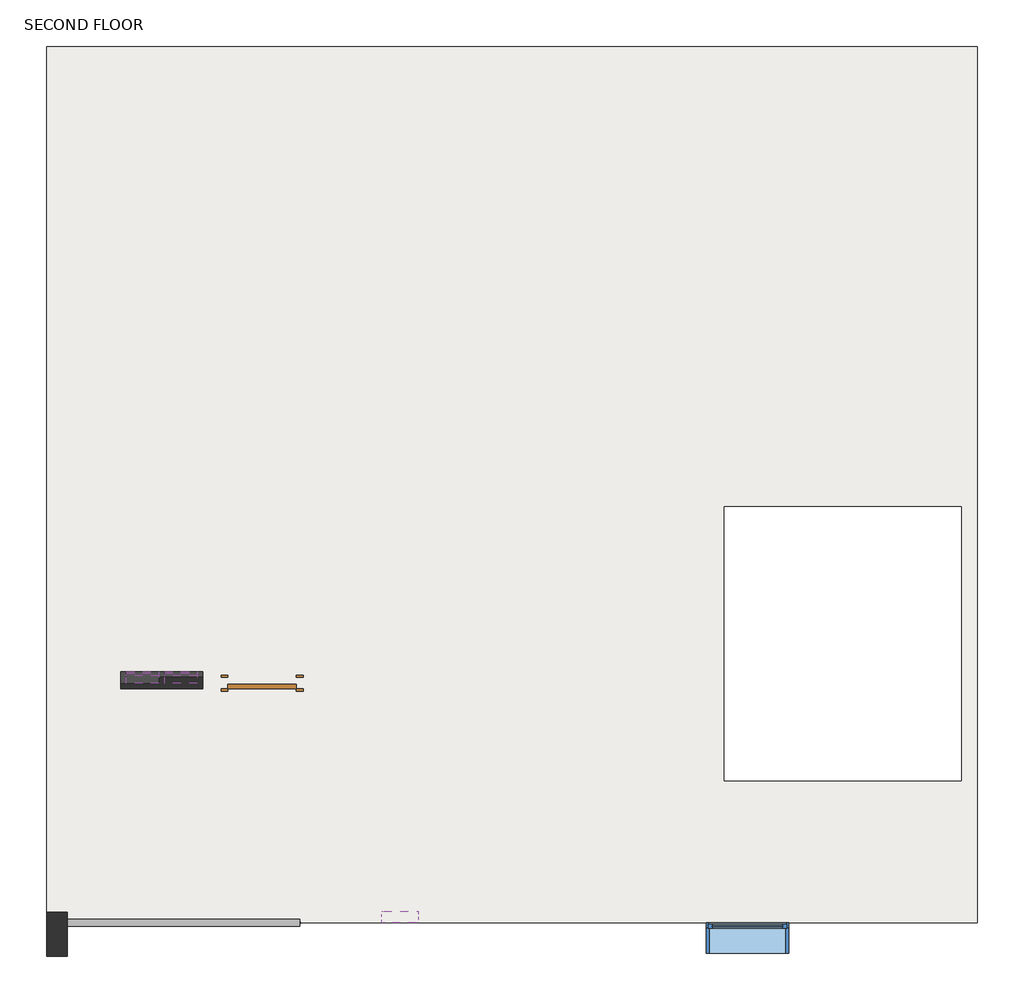
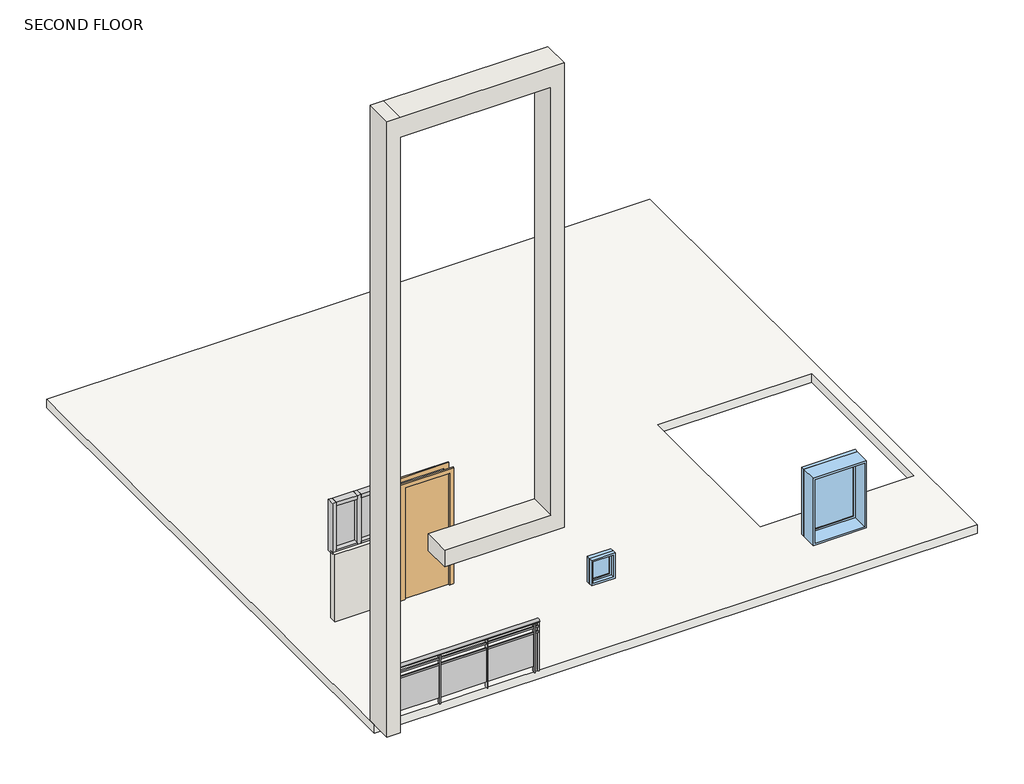
# One storey: 7 members, 2 plates, 2 walls, 2 windows, 1 door, 1 railing, 1 slab.
"""IFC4 building model written with IfcOpenShell, lengths in millimetres."""

from ifc_helpers import new_model, si_unit, point, frame, origin, place, context, project, spatial, polyline, ellipse_curve, trimmed, outline, extrude, transform, mapped, element, save
from ifc_brep_helpers import plane_surface, extruded_surface, advanced_brep
from components import door_e00f436c, member_d959a85f, member_843225dc, member_54f829b7, system_panel_glazed_8fc33089, walls_4_walls_4_370afa2d, fixed_bw_be0fa6e9, fixed_ven_0bde2124

model = new_model("IFC4")

# Units and contexts
model_context = context("Model", 3, world=origin())
ifc_project = project(units=[si_unit("LENGTHUNIT", "METRE", prefix="MILLI")], contexts=[model_context])

# Site, building, storey
site = spatial("IfcSite", under=ifc_project)
building = spatial("IfcBuilding", under=site)
storey = spatial("IfcBuildingStorey", under=building, Name="SECOND FLOOR", Elevation=6096.0)

# Door
placement = place(None, origin())
door_shape = door_e00f436c(model_context)
element("IfcDoor", 1, ObjectType="Single-Flush : 36\" x 84\"", at=placement, inside=storey, context=model_context, shape_type="MappedRepresentation", body=[
    mapped(door_shape, transform((-4124.5569651, 3118.5055142, 6096.0), x_axis=(1.0, 0.0, 0.0), y_axis=(0.0, 1.0, 0.0), z_axis=(0.0, 0.0, 1.0))),
])

# Members
member_shape = member_d959a85f(model_context)
element("IfcMember", 2, ObjectType="Rectangular Mullion : 2.5\" x 5\" rectangular", at=placement, inside=storey, context=model_context, shape_type="MappedRepresentation", body=[
    mapped(member_shape, transform((-4784.9569651, 3182.0055142, 7285.4584417), x_axis=(1.0, 0.0, 0.0), y_axis=(0.0, -1.0, 0.0), z_axis=(0.0, 0.0, -1.0))),
])
element("IfcMember", 3, ObjectType="Rectangular Mullion : 2.5\" x 5\" rectangular", at=placement, inside=storey, context=model_context, shape_type="MappedRepresentation", body=[
    mapped(member_shape, transform((-5699.3569651, 3182.0055142, 8204.2), x_axis=(-1.0, 0.0, 0.0), y_axis=(0.0, -1.0, 0.0), z_axis=(0.0, 0.0, 1.0))),
])
member_2_shape = member_843225dc(model_context)
element("IfcMember", 4, ObjectType="Rectangular Mullion : 2.5\" x 5\" rectangular", at=placement, inside=storey, context=model_context, shape_type="MappedRepresentation", body=[
    mapped(member_2_shape, transform((-4848.4569651, 3182.0055142, 8204.2), x_axis=(0.0, 0.0, 1.0), y_axis=(0.0, -1.0, 0.0), z_axis=(1.0, 0.0, 0.0))),
])
element("IfcMember", 5, ObjectType="Rectangular Mullion : 2.5\" x 5\" rectangular", at=placement, inside=storey, context=model_context, shape_type="MappedRepresentation", body=[
    mapped(member_2_shape, transform((-5273.9069651, 3182.0055142, 8204.2), x_axis=(0.0, 0.0, 1.0), y_axis=(0.0, -1.0, 0.0), z_axis=(1.0, 0.0, 0.0))),
])
element("IfcMember", 6, ObjectType="Rectangular Mullion : 2.5\" x 5\" rectangular", at=placement, inside=storey, context=model_context, shape_type="MappedRepresentation", body=[
    mapped(member_2_shape, transform((-5635.8569651, 3182.0055142, 7285.4584417), x_axis=(0.0, 0.0, -1.0), y_axis=(0.0, -1.0, 0.0), z_axis=(-1.0, 0.0, 0.0))),
])
element("IfcMember", 7, ObjectType="Rectangular Mullion : 2.5\" x 5\" rectangular", at=placement, inside=storey, context=model_context, shape_type="MappedRepresentation", body=[
    mapped(member_2_shape, transform((-5210.4069651, 3182.0055142, 7285.4584417), x_axis=(0.0, 0.0, -1.0), y_axis=(0.0, -1.0, 0.0), z_axis=(-1.0, 0.0, 0.0))),
])
member_3_shape = member_54f829b7(model_context)
element("IfcMember", 8, ObjectType="Rectangular Mullion : 2.5\" x 5\" rectangular", at=placement, inside=storey, context=model_context, shape_type="MappedRepresentation", body=[
    mapped(member_3_shape, transform((-5242.1569651, 3182.0055142, 7285.4584417), x_axis=(1.0, 0.0, 0.0), y_axis=(0.0, -1.0, 0.0), z_axis=(0.0, 0.0, -1.0))),
])

# Plates
system_panel_glazed_shape = system_panel_glazed_8fc33089(model_context)
element("IfcPlate", 9, ObjectType="System Panel : Glazed", at=placement, inside=storey, context=model_context, shape_type="MappedRepresentation", body=[
    mapped(system_panel_glazed_shape, transform((-5454.8819651, 3182.0055142, 7348.9584417), x_axis=(1.0, 0.0, 0.0), y_axis=(0.0, 1.0, 0.0), z_axis=(0.0, 0.0, 1.0))),
])
element("IfcPlate", 10, ObjectType="System Panel : Glazed", at=placement, inside=storey, context=model_context, shape_type="MappedRepresentation", body=[
    mapped(system_panel_glazed_shape, transform((-5029.4319651, 3182.0055142, 7348.9584417), x_axis=(1.0, 0.0, 0.0), y_axis=(0.0, 1.0, 0.0), z_axis=(0.0, 0.0, 1.0))),
])

# Railing
element("IfcRailing", 11, ObjectType="Glass Panel - Bottom Fill", at=placement, inside=storey, context=model_context, shape_type="SolidModel", body=[
    advanced_brep(
    [(-6296.2569651, 489.6055142, 7010.4), (-6296.2569651, 413.4055142, 7010.4), (-3705.4569651, 489.6055142, 7010.4), (-3705.4569651, 413.4055142, 7010.4)],
    [
        (0, 1, ellipse_curve(frame((-6296.2569651, 451.5055142, 7010.4), z_axis=(-1.0, 0.0, 0.0), x_axis=(0.0, -1.0, 0.0)), 38.1, 28.575)),
        (1, 0, ellipse_curve(frame((-6296.2569651, 451.5055142, 7010.4), z_axis=(-1.0, 0.0, 0.0), x_axis=(0.0, -1.0, 0.0)), 38.1, 28.575)),
        (2, 3, ellipse_curve(frame((-3705.4569651, 451.5055142, 7010.4), z_axis=(1.0, 0.0, 0.0), x_axis=(0.0, -1.0, 0.0)), 38.1, 28.575)),
        (3, 2, ellipse_curve(frame((-3705.4569651, 451.5055142, 7010.4), z_axis=(1.0, 0.0, 0.0), x_axis=(0.0, -1.0, 0.0)), 38.1, 28.575)),
        (0, 2),
        (3, 1),
    ],
    [
        plane_surface(frame((-6296.2569651, 451.5055142, 7010.4), z_axis=(-1.0, 0.0, 0.0), x_axis=(0.0, 1.0, 0.0))),
        plane_surface(frame((-3705.4569651, 451.5055142, 7010.4), z_axis=(1.0, 0.0, 0.0), x_axis=(0.0, 1.0, 0.0))),
        extruded_surface(trimmed(ellipse_curve(frame((-3705.4569651, 451.5055142, 7010.4), z_axis=(-1.0, 0.0, 0.0), x_axis=(0.0, -1.0, 0.0)), 38.1, 28.575), [point((-3705.4569651, 489.6055142, 7010.4))], [point((-3705.4569651, 413.4055142, 7010.4))], True, "CARTESIAN"), (-2590.8, 0.0, 0.0), 2590.8),
        extruded_surface(trimmed(ellipse_curve(frame((-3705.4569651, 451.5055142, 7010.4), z_axis=(-1.0, 0.0, 0.0), x_axis=(0.0, -1.0, 0.0)), 38.1, 28.575), [point((-3705.4569651, 413.4055142, 7010.4))], [point((-3705.4569651, 489.6055142, 7010.4))], True, "CARTESIAN"), (-2590.8, 0.0, 0.0), 2590.8),
    ],
    [
        (0, [[1, 2]]),
        (1, [[3, 4]]),
        (2, [[-1, 5, -4, 6]]),
        (3, [[-2, -6, -3, -5]]),
    ],
),
    extrude(outline(polyline([(-6296.2569651, 438.8055142), (-6296.2569651, 464.2055142), (-3705.4569651, 464.2055142), (-3705.4569651, 438.8055142), (-6296.2569651, 438.8055142)])), frame((0.0, 0.0, 6896.1), z_axis=(0.0, 0.0, 1.0), x_axis=(1.0, 0.0, 0.0)), (0.0, 0.0, 1.0), 25.4),
    extrude(outline(polyline([(-6296.2569651, 438.8055142), (-6296.2569651, 464.2055142), (-3705.4569651, 464.2055142), (-3705.4569651, 438.8055142), (-6296.2569651, 438.8055142)])), frame((0.0, 0.0, 6794.5), z_axis=(0.0, 0.0, 1.0), x_axis=(1.0, 0.0, 0.0)), (0.0, 0.0, 1.0), 25.4),
    extrude(outline(polyline([(-3788.0069651, 426.1055142), (-3788.0069651, 476.9055142), (-3775.3069651, 476.9055142), (-3775.3069651, 426.1055142), (-3788.0069651, 426.1055142)])), frame((0.0, 0.0, 6096.0), z_axis=(0.0, 0.0, 1.0), x_axis=(1.0, 0.0, 0.0)), (0.0, 0.0, 1.0), 885.6788223),
    extrude(outline(polyline([(-4594.4569651, 458.0406712), (-3781.6569651, 458.0406712), (-3781.6569651, 451.6906712), (-4594.4569651, 451.6906712), (-4594.4569651, 458.0406712)])), frame((0.0, 0.0, 6197.6), z_axis=(0.0, 0.0, 1.0), x_axis=(1.0, 0.0, 0.0)), (0.0, 0.0, 1.0), 596.9),
    extrude(outline(polyline([(-4600.8069651, 426.1055142), (-4600.8069651, 476.9055142), (-4588.1069651, 476.9055142), (-4588.1069651, 426.1055142), (-4600.8069651, 426.1055142)])), frame((0.0, 0.0, 6096.0), z_axis=(0.0, 0.0, 1.0), x_axis=(1.0, 0.0, 0.0)), (0.0, 0.0, 1.0), 885.6788223),
    extrude(outline(polyline([(-5407.2569651, 458.0406712), (-4594.4569651, 458.0406712), (-4594.4569651, 451.6906712), (-5407.2569651, 451.6906712), (-5407.2569651, 458.0406712)])), frame((0.0, 0.0, 6197.6), z_axis=(0.0, 0.0, 1.0), x_axis=(1.0, 0.0, 0.0)), (0.0, 0.0, 1.0), 596.9),
    extrude(outline(polyline([(-5413.6069651, 426.1055142), (-5413.6069651, 476.9055142), (-5400.9069651, 476.9055142), (-5400.9069651, 426.1055142), (-5413.6069651, 426.1055142)])), frame((0.0, 0.0, 6096.0), z_axis=(0.0, 0.0, 1.0), x_axis=(1.0, 0.0, 0.0)), (0.0, 0.0, 1.0), 885.6788223),
    extrude(outline(polyline([(-6220.0569651, 458.0406712), (-5407.2569651, 458.0406712), (-5407.2569651, 451.6906712), (-6220.0569651, 451.6906712), (-6220.0569651, 458.0406712)])), frame((0.0, 0.0, 6197.6), z_axis=(0.0, 0.0, 1.0), x_axis=(1.0, 0.0, 0.0)), (0.0, 0.0, 1.0), 596.9),
    extrude(outline(polyline([(-6226.4069651, 426.1055142), (-6226.4069651, 476.9055142), (-6213.7069651, 476.9055142), (-6213.7069651, 426.1055142), (-6226.4069651, 426.1055142)])), frame((0.0, 0.0, 6096.0), z_axis=(0.0, 0.0, 1.0), x_axis=(1.0, 0.0, 0.0)), (0.0, 0.0, 1.0), 885.6788223),
    extrude(outline(polyline([(-3718.1569651, 441.9805142), (-3718.1569651, 461.0305142), (-3699.1069651, 461.0305142), (-3699.1069651, 441.9805142), (-3718.1569651, 441.9805142)])), frame((0.0, 0.0, 6096.0), z_axis=(0.0, 0.0, 1.0), x_axis=(1.0, 0.0, 0.0)), (0.0, 0.0, 1.0), 885.6788223),
    extrude(outline(polyline([(-6302.6069651, 441.9805142), (-6302.6069651, 461.0305142), (-6283.5569651, 461.0305142), (-6283.5569651, 441.9805142), (-6302.6069651, 441.9805142)])), frame((0.0, 0.0, 6096.0), z_axis=(0.0, 0.0, 1.0), x_axis=(1.0, 0.0, 0.0)), (0.0, 0.0, 1.0), 885.6788223),
])

# Slab
element("IfcSlab", 12, ObjectType="Generic - 12\"", at=placement, inside=storey, context=model_context, shape_type="SweptSolid", body=[
    extrude(outline(polyline([(3838.3430349, 10205.1055142), (3838.3430349, 451.5055142), (-6524.8569651, 451.5055142), (-6524.8569651, 10205.1055142), (3838.3430349, 10205.1055142)]), holes=[polyline([(3660.5430349, 5080.6555142), (1018.9430349, 5080.6555142), (1018.9430349, 2032.6555142), (3660.5430349, 2032.6555142), (3660.5430349, 5080.6555142)])]), frame((0.0, 0.0, 5943.6), z_axis=(0.0, 0.0, 1.0), x_axis=(1.0, 0.0, 0.0)), (0.0, 0.0, 1.0), 152.4),
])

# Walls
element("IfcWall", 13, ObjectType="5\"", at=placement, inside=storey, context=model_context, shape_type="SweptSolid", body=[
    extrude(outline(polyline([(-4784.9569651, 3055.0055142), (-5699.3569651, 3055.0055142), (-5699.3569651, 3182.0055142), (-4784.9569651, 3182.0055142), (-4784.9569651, 3055.0055142)])), frame((0.0, 0.0, 5156.2), z_axis=(0.0, 0.0, 1.0), x_axis=(1.0, 0.0, 0.0)), (0.0, 0.0, 1.0), 2159.0),
])
walls_4_walls_4_shape = walls_4_walls_4_370afa2d(model_context)
element("IfcWall", 14, ObjectType="Walls 4 : Walls 4", at=placement, inside=storey, context=model_context, shape_type="MappedRepresentation", body=[
    mapped(walls_4_walls_4_shape, transform((0.0, 0.0, 0.0), x_axis=(1.0, 0.0, 0.0), y_axis=(0.0, 1.0, 0.0), z_axis=(0.0, 0.0, 1.0))),
])

# Windows
fixed_bw_shape = fixed_bw_be0fa6e9(model_context)
element("IfcWindow", 15, ObjectType="Fixed : BW", at=placement, inside=storey, context=model_context, shape_type="MappedRepresentation", body=[
    mapped(fixed_bw_shape, transform((1316.0073388, 281.3921573, 6070.6), x_axis=(1.0, 0.0, 0.0), y_axis=(0.0, 1.0, 0.0), z_axis=(0.0, 0.0, 1.0))),
])
fixed_ven_shape = fixed_ven_0bde2124(model_context)
element("IfcWindow", 16, ObjectType="Fixed : VEN", at=placement, inside=storey, context=model_context, shape_type="MappedRepresentation", body=[
    mapped(fixed_ven_shape, transform((-2549.7569651, 515.0055142, 6397.0646104), x_axis=(1.0, 0.0, 0.0), y_axis=(0.0, 1.0, 0.0), z_axis=(0.0, 0.0, 1.0))),
])

save(model, "model.ifc")

# Revit data of these elements
# Type "Single-Flush : 36\" x 84\""
#   Type Mark = "1"
#   Construction Type Id = "MDOOR"
#   Assembly Code = "C1020"
#   Analytic Construction = "Metal"
#   Thickness = 0' - 2"
#   Heat Transfer Coefficient (U) = 0.651978 BTU/(h·ft²·°F)
#   Height = 6' - 8"
#   Trim Projection Ext = 0' - 1"
#   Trim Projection Int = 0' - 1"
#   Trim Width = 0' - 3"
#   Width = 2' - 6"
#   Define Thermal Properties by = 1
#   Define Thermal Properties by = 1
#   Door Material = Door - Panel
#   Frame Material = Door - Frame
#   Visual Light Transmittance = 0
#   Solar Heat Gain Coefficient = 0
#   Function = (empty or 0)
#   Wall Closure = (empty or 0)
# Type "Rectangular Mullion : 2.5\" x 5\" rectangular"
#   built-in parameter 1007304 = 0.416667 (stored number, unit not read)
#   built-in parameter 1007301 = 0.104167 (stored number, unit not read)
#   built-in parameter 1007300 = 0.104167 (stored number, unit not read)
# Type "System Panel : Glazed"
#   Construction Type Id = "GSP4R"
#   Analytic Construction = "1/8 in Pilkington single glazing"
#   Visual Light Transmittance = 0.9
#   Solar Heat Gain Coefficient = 0.86
#   Heat Transfer Coefficient (U) = 1.18115 BTU/(h·ft²·°F)
#   Define Thermal Properties by = 1
# Type "Glass Panel - Bottom Fill"
#   Assembly Code = "C2010400"
#   built-in parameter 1008612 = 0.0416667 (stored number, unit not read)
#   built-in parameter 1008611 = 0.0416667 (stored number, unit not read)
#   built-in parameter 1008609 = 0.333333 (stored number, unit not read)
#   built-in parameter 1008604 = 0.166667 (stored number, unit not read)
#   built-in parameter 1008603 = 0.166667 (stored number, unit not read)
#   Railing Height = 3' - 0"
#   built-in parameter 1008630 = 2
#   built-in parameter 1008610 = 2
#   built-in parameter 1008618 = Baluster - Square : 3/4"
# Type "Generic - 12\""
#   Assembly Code = "B1010"
#   Function = 0
#   Layers, outside or top first: 0' - 6" no material (function 1)
# Type "5\""
#   Assembly Code = "B2010"
#   Layers, outside or top first: 0' - 5" "Concrete Masonry Units" (function 1)
# Type "Fixed : BW"
#   Type Mark = "18"
#   Construction Type Id = "GSP4R"
#   Assembly Code = "B2020100"
#   Analytic Construction = "1/8 in Pilkington single glazing"
#   Visual Light Transmittance = 0.9
#   Solar Heat Gain Coefficient = 0.78
#   Heat Transfer Coefficient (U) = 0.6496 BTU/(h·ft²·°F)
#   Height = 4' - 0"
#   Default Sill Height = 3' - 0"
#   Width = 3' - 0"
#   Window Inset = 0' - 0 3/4"
#   Define Thermal Properties by = 1
#   Glass Pane Material = Glass
#   Sash Material = Sash
#   Wall Closure = (empty or 0)
# Type "Fixed : VEN"
#   Type Mark = "19"
#   Construction Type Id = "GSP4R"
#   Assembly Code = "B2020100"
#   Analytic Construction = "1/8 in Pilkington single glazing"
#   Visual Light Transmittance = 0.9
#   Solar Heat Gain Coefficient = 0.78
#   Heat Transfer Coefficient (U) = 0.6496 BTU/(h·ft²·°F)
#   Height = 1' - 6"
#   Default Sill Height = 3' - 0"
#   Width = 1' - 4"
#   Window Inset = 0' - 0 3/4"
#   Define Thermal Properties by = 1
#   Glass Pane Material = Glass
#   Sash Material = Sash
#   Wall Closure = (empty or 0)
# Element 1 (IfcDoor, "Single-Flush : 36\" x 84\"")
#   Phase Created = New Construction
#   Materials on its faces: "Door - Frame", "Door - Panel"
# Elements 2, 3, 4, 5, 6, 7, 8 (IfcMember, "Rectangular Mullion : 2.5\" x 5\" rectangular")
#   Phase Created = New Construction
#   Materials on its faces: "Aluminum"
# Elements 9, 10 (IfcPlate, "System Panel : Glazed")
#   Phase Created = New Construction
#   Materials on its faces: "Glass"
# Element 11 (IfcRailing, "Glass Panel - Bottom Fill")
#   Phase Created = New Construction
#   Materials on its faces: "Glass"
# Element 12 (IfcSlab, "Generic - 12\"")
#   Height Offset From Level = 0' - 0"
#   Phase Created = New Construction
#   Materials on its faces: "Default Floor", "1 wall brown"
# Element 13 (IfcWall, "5\"")
#   built-in parameter 1001111 = -3' - 1"
#   Top Offset = 0' - 0"
#   Base Offset = -3' - 1"
#   Unconnected Height = 7' - 1"
#   wall height = 7' - 1"
#   Phase Created = New Construction
#   Base Constraint = SECOND FLOOR
#   Materials on its faces: "Concrete Masonry Units", "1 wall white"
# Element 14 (IfcWall, "Walls 4 : Walls 4")
#   Phase Created = New Construction
#   Materials on its faces: "1 wall brown", "Default Wall"
# Element 15 (IfcWindow, "Fixed : BW")
#   Mark = "8"
#   Phase Created = New Construction
#   Materials on its faces: "Sash", "Glass"
# Element 16 (IfcWindow, "Fixed : VEN")
#   Mark = "11"
#   Phase Created = New Construction
#   Materials on its faces: "Sash", "Glass"
# Materials
#   "Door - Panel": class "Wood", colour RGB 210 159 95, transparency 0, Cost = 0
#   "Door - Frame": colour RGB 118 70 51, transparency 0, Cost = 0
#   "Concrete Masonry Units": class "Masonry", colour RGB 227 227 227, transparency 0, Description = "Concrete masonry units", Cost = 0
#   "Glass": class "Glass", colour RGB 0 128 192, transparency 0.75, Description = "Soda Lime Glass", Cost = 0
#   "Sash": class "Wood", colour RGB 224 178 126, transparency 0, Cost = 0
#   "Aluminum": class "Metal", colour RGB 247 247 247, transparency 0, Description = "Aluminum 6061", Cost = 0
#   "Default Floor": colour RGB 128 128 128, transparency 0, Cost = 0
#   "1 wall brown": class "Generic", colour RGB 61 46 37, transparency 0, Cost = 0
#   "1 wall white": class "Generic", colour RGB 244 245 241, transparency 0, Cost = 0
#   "Default Wall": colour RGB 128 128 128, transparency 0, Cost = 0
